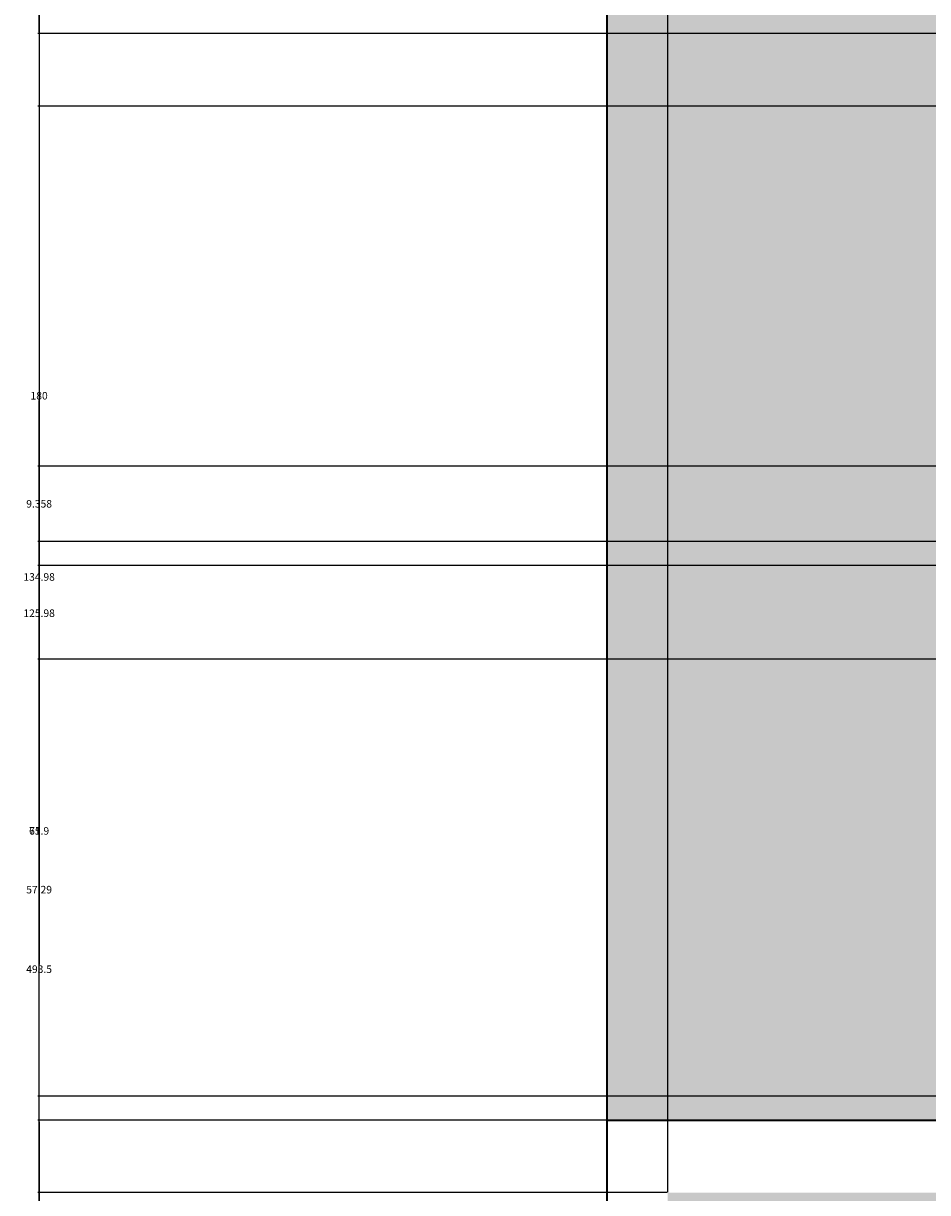
# Model space of a CAD drawing. Units: inches. Extents: x -5 to 714, y 84 to 644.
# Tile 7 of 20: x -5 to 108, y 336 to 481. Entities that reach past the tile are written whole.
import ezdxf

# ---------------------------------------------------------------- set-up
doc = ezdxf.new("R2010")
doc.units = ezdxf.units.IN
doc.header["$MEASUREMENT"] = 0
for name, color, linetype, lineweight in [('A-ANNO-DIMS', 2, 'Continuous', 18), ('A-ELEV', 7, 'Continuous', 35), ('A-ELEV-PATT', 8, 'Continuous', 13)]:
    doc.layers.add(name, color=color, linetype=linetype, lineweight=lineweight)
doc.styles.get("Standard").update_dxf_attribs({"font": 'arial.ttf'})
doc.dimstyles.get("Standard").update_dxf_attribs({"dimtxt": 0.9375, "dimasz": 0.18, "dimexe": 0.18, "dimexo": 0.0625, "dimgap": 0.09, "dimtad": 0, "dimtih": 1, "dimtoh": 1, "dimdec": 4, "dimzin": 0, "dimdsep": 46, "dimlunit": 4, "dimtxsty": 'Standard', "dimcen": 0.09, "dimadec": 0, "dimazin": 0, "dimtfac": 1, "dimtdec": 4, "dimtofl": 0, "dimtmove": 0, "dimatfit": 3, "dimfxl": 1, "dimtolj": 1, "dimtzin": 0, "dimarcsym": 0})

# ---------------------------------------------------------------- blocks, each defined once
blk = doc.blocks.new('*D2')
at = {"layer": 'A-ANNO-DIMS', "color": 0, "lineweight": -2, "transparency": 16777216}
for p, q in [((67.93, 610.73), (-2.74, 610.73)), ((-2.56, 610.55), (-2.56, 364.53)), ((-2.56, 117.37), (-2.56, 363.39)), ((30.08, 117.19), (-2.74, 117.19))]:
    blk.add_line(p, q, dxfattribs=at)
at = {"layer": 'A-ANNO-DIMS', "color": 0, "transparency": 16777216}
for points in [[(-2.59, 610.55), (-2.53, 610.55), (-2.56, 610.73)], [(-2.59, 117.37), (-2.53, 117.37), (-2.56, 117.19)]]:
    blk.add_solid(points, dxfattribs=at)
at = {"layer": 'Defpoints', "color": 0, "transparency": 16777216}
for p in [(-2.56, 610.73), (67.99, 610.73), (30.14, 117.19)]:
    blk.add_point(p, dxfattribs=at)
at = {"layer": 'A-ANNO-DIMS', "color": 0, "transparency": 16777216, "insert": (-2.56, 363.96), "char_height": 0.938, "attachment_point": 5}
blk.add_mtext('\\A1;493.5', dxfattribs=at)
blk = doc.blocks.new('*D5')
at = {"layer": 'A-ANNO-DIMS', "color": 0, "lineweight": -2, "transparency": 16777216}
for p, q in [((67.93, 345.19), (-2.74, 345.19)), ((-2.56, 345.01), (-2.56, 273.75)), ((-2.56, 201.37), (-2.56, 272.63)), ((67.93, 201.19), (-2.74, 201.19))]:
    blk.add_line(p, q, dxfattribs=at)
at = {"layer": 'A-ANNO-DIMS', "color": 0, "transparency": 16777216}
for points in [[(-2.59, 345.01), (-2.53, 345.01), (-2.56, 345.19)], [(-2.59, 201.37), (-2.53, 201.37), (-2.56, 201.19)]]:
    blk.add_solid(points, dxfattribs=at)
at = {"layer": 'Defpoints', "color": 0, "transparency": 16777216}
for p in [(-2.56, 345.19), (67.99, 345.19), (67.99, 201.19)]:
    blk.add_point(p, dxfattribs=at)
at = {"layer": 'A-ANNO-DIMS', "color": 0, "transparency": 16777216, "insert": (-2.56, 273.19), "char_height": 0.938, "attachment_point": 5}
blk.add_mtext('\\A1;144', dxfattribs=at)
blk = doc.blocks.new('*D6')
at = {"layer": 'A-ANNO-DIMS', "color": 0, "lineweight": -2, "transparency": 16777216}
for p, q in [((67.93, 525.19), (-2.74, 525.19)), ((-2.56, 525.01), (-2.56, 435.76)), ((-2.56, 345.37), (-2.56, 434.62)), ((67.93, 345.19), (-2.74, 345.19))]:
    blk.add_line(p, q, dxfattribs=at)
at = {"layer": 'A-ANNO-DIMS', "color": 0, "transparency": 16777216}
for points in [[(-2.59, 525.01), (-2.53, 525.01), (-2.56, 525.19)], [(-2.59, 345.37), (-2.53, 345.37), (-2.56, 345.19)]]:
    blk.add_solid(points, dxfattribs=at)
at = {"layer": 'Defpoints', "color": 0, "transparency": 16777216}
for p in [(-2.56, 525.19), (67.99, 525.19), (67.99, 345.19)]:
    blk.add_point(p, dxfattribs=at)
at = {"layer": 'A-ANNO-DIMS', "color": 0, "transparency": 16777216, "insert": (-2.56, 435.19), "char_height": 0.938, "attachment_point": 5}
blk.add_mtext('\\A1;180', dxfattribs=at)
blk = doc.blocks.new('*D16')
at = {"layer": 'A-ANNO-DIMS', "color": 0, "lineweight": -2, "transparency": 16777216}
for p, q in [((364.22, 540.29), (-2.74, 540.29)), ((-2.56, 540.11), (-2.56, 510.8)), ((-2.56, 480.35), (-2.56, 509.66)), ((364.22, 480.17), (-2.74, 480.17))]:
    blk.add_line(p, q, dxfattribs=at)
at = {"layer": 'A-ANNO-DIMS', "color": 0, "transparency": 16777216}
for points in [[(-2.59, 540.11), (-2.53, 540.11), (-2.56, 540.29)], [(-2.59, 480.35), (-2.53, 480.35), (-2.56, 480.17)]]:
    blk.add_solid(points, dxfattribs=at)
at = {"layer": 'Defpoints', "color": 0, "transparency": 16777216}
for p in [(-2.56, 540.29), (364.28, 540.29), (364.28, 480.17)]:
    blk.add_point(p, dxfattribs=at)
at = {"layer": 'A-ANNO-DIMS', "color": 0, "transparency": 16777216, "insert": (-2.56, 510.23), "char_height": 0.938, "attachment_point": 5}
blk.add_mtext('\\A1;60.11', dxfattribs=at)
blk = doc.blocks.new('*D23')
at = {"layer": 'A-ANNO-DIMS', "color": 0, "lineweight": -2, "transparency": 16777216}
for p, q in [((229.3, 525.19), (-2.74, 525.19)), ((-2.56, 525.01), (-2.56, 503.25)), ((-2.56, 480.35), (-2.56, 502.11)), ((229.3, 480.17), (-2.74, 480.17))]:
    blk.add_line(p, q, dxfattribs=at)
at = {"layer": 'A-ANNO-DIMS', "color": 0, "transparency": 16777216}
for points in [[(-2.59, 525.01), (-2.53, 525.01), (-2.56, 525.19)], [(-2.59, 480.35), (-2.53, 480.35), (-2.56, 480.17)]]:
    blk.add_solid(points, dxfattribs=at)
at = {"layer": 'Defpoints', "color": 0, "transparency": 16777216}
for p in [(-2.56, 525.19), (229.36, 525.19), (229.36, 480.17)]:
    blk.add_point(p, dxfattribs=at)
at = {"layer": 'A-ANNO-DIMS', "color": 0, "transparency": 16777216, "insert": (-2.56, 502.68), "char_height": 0.938, "attachment_point": 5}
blk.add_mtext('\\A1;45.02', dxfattribs=at)
blk = doc.blocks.new('*D25')
at = {"layer": 'A-ANNO-DIMS', "color": 0, "lineweight": -2, "transparency": 16777216}
for p, q in [((126.67, 480.17), (-2.74, 480.17)), ((-2.56, 479.99), (-2.56, 413.25)), ((-2.56, 345.37), (-2.56, 412.11)), ((126.67, 345.19), (-2.74, 345.19))]:
    blk.add_line(p, q, dxfattribs=at)
at = {"layer": 'A-ANNO-DIMS', "color": 0, "transparency": 16777216}
for points in [[(-2.59, 479.99), (-2.53, 479.99), (-2.56, 480.17)], [(-2.59, 345.37), (-2.53, 345.37), (-2.56, 345.19)]]:
    blk.add_solid(points, dxfattribs=at)
at = {"layer": 'Defpoints', "color": 0, "transparency": 16777216}
for p in [(-2.56, 480.17), (126.73, 480.17), (126.73, 345.19)]:
    blk.add_point(p, dxfattribs=at)
at = {"layer": 'A-ANNO-DIMS', "color": 0, "transparency": 16777216, "insert": (-2.56, 412.68), "char_height": 0.938, "attachment_point": 5}
blk.add_mtext('\\A1;134.98', dxfattribs=at)
blk = doc.blocks.new('*D26')
at = {"layer": 'A-ANNO-DIMS', "color": 0, "lineweight": -2, "transparency": 16777216}
for p, q in [((135.67, 471.17), (-2.74, 471.17)), ((-2.56, 470.99), (-2.56, 408.75)), ((-2.56, 345.37), (-2.56, 407.61)), ((135.67, 345.19), (-2.74, 345.19))]:
    blk.add_line(p, q, dxfattribs=at)
at = {"layer": 'A-ANNO-DIMS', "color": 0, "transparency": 16777216}
for points in [[(-2.59, 470.99), (-2.53, 470.99), (-2.56, 471.17)], [(-2.59, 345.37), (-2.53, 345.37), (-2.56, 345.19)]]:
    blk.add_solid(points, dxfattribs=at)
at = {"layer": 'Defpoints', "color": 0, "transparency": 16777216}
for p in [(-2.56, 471.17), (135.73, 471.17), (135.73, 345.19)]:
    blk.add_point(p, dxfattribs=at)
at = {"layer": 'A-ANNO-DIMS', "color": 0, "transparency": 16777216, "insert": (-2.56, 408.18), "char_height": 0.938, "attachment_point": 5}
blk.add_mtext('\\A1;125.98', dxfattribs=at)
blk = doc.blocks.new('*D27')
at = {"layer": 'A-ANNO-DIMS', "color": 0, "lineweight": -2, "transparency": 16777216}
for p, q in [((429.45, 402.48), (-2.74, 402.48)), ((-2.56, 402.3), (-2.56, 374.41)), ((-2.56, 345.37), (-2.56, 373.27)), ((429.45, 345.19), (-2.74, 345.19))]:
    blk.add_line(p, q, dxfattribs=at)
at = {"layer": 'A-ANNO-DIMS', "color": 0, "transparency": 16777216}
for points in [[(-2.59, 402.3), (-2.53, 402.3), (-2.56, 402.48)], [(-2.59, 345.37), (-2.53, 345.37), (-2.56, 345.19)]]:
    blk.add_solid(points, dxfattribs=at)
at = {"layer": 'Defpoints', "color": 0, "transparency": 16777216}
for p in [(-2.56, 402.48), (429.51, 402.48), (429.51, 345.19)]:
    blk.add_point(p, dxfattribs=at)
at = {"layer": 'A-ANNO-DIMS', "color": 0, "transparency": 16777216, "insert": (-2.56, 373.84), "char_height": 0.938, "attachment_point": 5}
blk.add_mtext('\\A1;57.29', dxfattribs=at)
blk = doc.blocks.new('*D34')
at = {"layer": 'A-ANNO-DIMS', "color": 0, "lineweight": -2, "transparency": 16777216}
for p, q in [((286.82, 414.09), (-2.74, 414.09)), ((-2.56, 413.91), (-2.56, 381.71)), ((-2.56, 348.37), (-2.56, 380.57)), ((286.82, 348.19), (-2.74, 348.19))]:
    blk.add_line(p, q, dxfattribs=at)
at = {"layer": 'A-ANNO-DIMS', "color": 0, "transparency": 16777216}
for points in [[(-2.59, 413.91), (-2.53, 413.91), (-2.56, 414.09)], [(-2.59, 348.37), (-2.53, 348.37), (-2.56, 348.19)]]:
    blk.add_solid(points, dxfattribs=at)
at = {"layer": 'Defpoints', "color": 0, "transparency": 16777216}
for p in [(-2.56, 414.09), (286.88, 414.09), (286.88, 348.19)]:
    blk.add_point(p, dxfattribs=at)
at = {"layer": 'A-ANNO-DIMS', "color": 0, "transparency": 16777216, "insert": (-2.56, 381.14), "char_height": 0.938, "attachment_point": 5}
blk.add_mtext('\\A1;65.9', dxfattribs=at)
blk = doc.blocks.new('*D35')
at = {"layer": 'A-ANNO-DIMS', "color": 0, "lineweight": -2, "transparency": 16777216}
for p, q in [((289.82, 417.09), (-2.74, 417.09)), ((-2.56, 416.91), (-2.56, 381.71)), ((-2.56, 345.37), (-2.56, 380.57)), ((289.82, 345.19), (-2.74, 345.19))]:
    blk.add_line(p, q, dxfattribs=at)
at = {"layer": 'A-ANNO-DIMS', "color": 0, "transparency": 16777216}
for points in [[(-2.59, 416.91), (-2.53, 416.91), (-2.56, 417.09)], [(-2.59, 345.37), (-2.53, 345.37), (-2.56, 345.19)]]:
    blk.add_solid(points, dxfattribs=at)
at = {"layer": 'Defpoints', "color": 0, "transparency": 16777216}
for p in [(-2.56, 417.09), (289.88, 417.09), (289.88, 345.19)]:
    blk.add_point(p, dxfattribs=at)
at = {"layer": 'A-ANNO-DIMS', "color": 0, "transparency": 16777216, "insert": (-2.56, 381.14), "char_height": 0.938, "attachment_point": 5}
blk.add_mtext('\\A1;71.9', dxfattribs=at)
blk = doc.blocks.new('*D37')
at = {"layer": 'A-ANNO-DIMS', "color": 0, "lineweight": -2, "transparency": 16777216}
for p, q in [((302.44, 426.45), (-2.74, 426.45)), ((-2.56, 426.27), (-2.56, 422.34)), ((-2.56, 417.27), (-2.56, 421.2)), ((302.44, 417.09), (-2.74, 417.09))]:
    blk.add_line(p, q, dxfattribs=at)
at = {"layer": 'A-ANNO-DIMS', "color": 0, "transparency": 16777216}
for points in [[(-2.59, 426.27), (-2.53, 426.27), (-2.56, 426.45)], [(-2.59, 417.27), (-2.53, 417.27), (-2.56, 417.09)]]:
    blk.add_solid(points, dxfattribs=at)
at = {"layer": 'Defpoints', "color": 0, "transparency": 16777216}
for p in [(-2.56, 426.45), (302.5, 426.45), (302.5, 417.09)]:
    blk.add_point(p, dxfattribs=at)
at = {"layer": 'A-ANNO-DIMS', "color": 0, "transparency": 16777216, "insert": (-2.56, 421.77), "char_height": 0.938, "attachment_point": 5}
blk.add_mtext('\\A1;9.358', dxfattribs=at)
blk = doc.blocks.new('*D45')
at = {"layer": 'A-ANNO-DIMS', "color": 0, "lineweight": -2, "transparency": 16777216}
for p, q in [((75.44, 336.21), (-2.74, 336.21)), ((-2.56, 336.03), (-2.56, 328.34)), ((-2.56, 319.52), (-2.56, 327.21)), ((75.44, 319.34), (-2.74, 319.34))]:
    blk.add_line(p, q, dxfattribs=at)
at = {"layer": 'A-ANNO-DIMS', "color": 0, "transparency": 16777216}
for points in [[(-2.59, 336.03), (-2.53, 336.03), (-2.56, 336.21)], [(-2.59, 319.52), (-2.53, 319.52), (-2.56, 319.34)]]:
    blk.add_solid(points, dxfattribs=at)
at = {"layer": 'Defpoints', "color": 0, "transparency": 16777216}
for p in [(-2.56, 336.21), (75.5, 336.21), (75.5, 319.34)]:
    blk.add_point(p, dxfattribs=at)
at = {"layer": 'A-ANNO-DIMS', "color": 0, "transparency": 16777216, "insert": (-2.56, 327.78), "char_height": 0.938, "attachment_point": 5}
blk.add_mtext('\\A1;16.86', dxfattribs=at)
blk = doc.blocks.new('*D46')
at = {"layer": 'A-ANNO-DIMS', "color": 0, "lineweight": -2, "transparency": 16777216}
for p, q in [((67.99, 345.26), (67.99, 643.61)), ((68.17, 643.43), (70.08, 643.43)), ((75.32, 643.43), (73.41, 643.43)), ((75.5, 336.27), (75.5, 643.61))]:
    blk.add_line(p, q, dxfattribs=at)
at = {"layer": 'A-ANNO-DIMS', "color": 0, "transparency": 16777216}
for points in [[(68.17, 643.46), (68.17, 643.4), (67.99, 643.43)], [(75.32, 643.46), (75.32, 643.4), (75.5, 643.43)]]:
    blk.add_solid(points, dxfattribs=at)
at = {"layer": 'Defpoints', "color": 0, "transparency": 16777216}
for p in [(75.5, 643.43), (67.99, 345.19), (75.5, 336.21)]:
    blk.add_point(p, dxfattribs=at)
at = {"layer": 'A-ANNO-DIMS', "color": 0, "transparency": 16777216, "insert": (71.75, 643.43), "char_height": 0.938, "attachment_point": 5}
blk.add_mtext('\\A1;7.516', dxfattribs=at)
blk = doc.blocks.new('*D47')
at = {"layer": 'A-ANNO-DIMS', "color": 0, "lineweight": -2, "transparency": 16777216}
for p, q in [((75.5, 336.27), (75.5, 643.61)), ((75.68, 643.43), (96.74, 643.43)), ((121.18, 643.43), (100.13, 643.43)), ((121.36, 336.27), (121.36, 643.61))]:
    blk.add_line(p, q, dxfattribs=at)
at = {"layer": 'A-ANNO-DIMS', "color": 0, "transparency": 16777216}
for points in [[(75.68, 643.46), (75.68, 643.4), (75.5, 643.43)], [(121.18, 643.46), (121.18, 643.4), (121.36, 643.43)]]:
    blk.add_solid(points, dxfattribs=at)
at = {"layer": 'Defpoints', "color": 0, "transparency": 16777216}
for p in [(121.36, 643.43), (75.5, 336.21), (121.36, 336.21)]:
    blk.add_point(p, dxfattribs=at)
at = {"layer": 'A-ANNO-DIMS', "color": 0, "transparency": 16777216, "insert": (98.43, 643.43), "char_height": 0.938, "attachment_point": 5}
blk.add_mtext('\\A1;45.85', dxfattribs=at)
blk = doc.blocks.new('*D50')
at = {"layer": 'A-ANNO-DIMS', "color": 0, "lineweight": -2, "transparency": 16777216}
for p, q in [((200.67, 345.19), (-2.74, 345.19)), ((-2.56, 345.01), (-2.56, 324.13)), ((-2.56, 302.12), (-2.56, 323)), ((200.67, 301.94), (-2.74, 301.94))]:
    blk.add_line(p, q, dxfattribs=at)
at = {"layer": 'A-ANNO-DIMS', "color": 0, "transparency": 16777216}
for points in [[(-2.59, 345.01), (-2.53, 345.01), (-2.56, 345.19)], [(-2.59, 302.12), (-2.53, 302.12), (-2.56, 301.94)]]:
    blk.add_solid(points, dxfattribs=at)
at = {"layer": 'Defpoints', "color": 0, "transparency": 16777216}
for p in [(-2.56, 345.19), (200.74, 345.19), (200.74, 301.94)]:
    blk.add_point(p, dxfattribs=at)
at = {"layer": 'A-ANNO-DIMS', "color": 0, "transparency": 16777216, "insert": (-2.56, 323.57), "char_height": 0.938, "attachment_point": 5}
blk.add_mtext('\\A1;43.255', dxfattribs=at)

msp = doc.modelspace()

# ---------------------------------------------------------------- hatches: boundary and pattern name
at = {"layer": 'A-ELEV-PATT', "transparency": 33554687}
h = msp.add_hatch(color=256, dxfattribs=at)
h.dxf.hatch_style = 1
h.paths.add_polyline_path([(188.3677, 525.1928), (67.9893, 525.1928), (67.9893, 489.1928), (67.9893, 345.1928), (126.7303, 345.1928), (126.7303, 480.1709), (229.3575, 480.1709), (229.3575, 525.1928), (212.6043, 525.1928), (212.6043, 482.7164), (211.0019, 482.7164), (211.0019, 525.1928), (207.6919, 525.1928), (199.9852, 525.1928), (199.9852, 482.7164), (198.3828, 482.7164), (198.3828, 525.1928), (189.9701, 525.1928), (189.9701, 482.7164), (188.3677, 482.7164)])
h.paths.add_polyline_path([(121.3589, 336.2066), (75.5048, 336.2066), (75.5048, 319.345), (121.3589, 319.345)])
h.paths.add_polyline_path([(121.3589, 319.345), (75.5048, 319.345), (75.5048, 302.3045), (121.3589, 302.3045)])
h.paths.add_polyline_path([(121.3589, 302.3045), (75.5048, 302.3045), (75.5048, 282.8561), (121.3589, 282.8561)])
h.paths.add_polyline_path([(121.3589, 282.8561), (75.5048, 282.8561), (75.5048, 261.5556), (121.3589, 261.5556)])
h.paths.add_polyline_path([(121.3589, 261.5556), (75.5048, 261.5556), (75.5048, 243.7009), (121.3589, 243.7009)])
h.paths.add_polyline_path([(121.3589, 243.7009), (75.5048, 243.7009), (75.5048, 223.5117), (121.3589, 223.5117)])
h.paths.add_polyline_path([(121.3589, 223.5117), (75.5048, 223.5117), (75.5048, 212.5836), (121.3589, 212.5836)])
h.paths.add_polyline_path([(121.3589, 212.5836), (75.5048, 212.5836), (75.5048, 201.1928), (121.3589, 201.1928)])
h.paths.add_polyline_path([(179.9335, 201.1928), (30.1395, 201.1928), (30.1395, 198.7054), (179.9335, 198.7054)])
h.paths.add_polyline_path([(187.6349, 201.1928), (179.9335, 201.1928), (179.9335, 198.7054), (179.9335, 141.1928), (269.2446, 141.1928), (269.2446, 201.1928), (263.4349, 201.1928), (263.4349, 152.1176), (187.6349, 152.1176)])
h.paths.add_polyline_path([(269.2446, 277.0513), (269.2446, 287.501), (269.2446, 306.6286), (578.0915, 306.6286), (578.0915, 201.1928), (593.428, 201.1928), (593.428, 315.0968), (584.4202, 315.0968), (259.0665, 315.0968), (259.0665, 201.1928), (263.4349, 201.1928), (269.2446, 201.1928)])

# ---------------------------------------------------------------- linework, layer by layer
at = {"layer": 'A-ELEV'}
for p, q in [((67.9893, 345.1928), (67.9893, 489.1928)), ((67.9893, 201.1928), (67.9893, 345.1928)), ((67.9893, 345.1928), (587.5794, 345.1928))]:
    msp.add_line(p, q, dxfattribs=at)

# ---------------------------------------------------------------- dimensions: what is measured, and where the dimension line sits
at = {"layer": 'A-ANNO-DIMS'}
for base, p1, p2, override, picture, middle in [((75.50483, 643.42757), (67.9893, 345.19283), (75.50483, 336.20661), {"dimdec": 3, "dimlfac": 1, "dimrnd": 0, "dimzin": 0, "dimdsep": 46, "dimlunit": 2}, '*D46', (71.74706, 643.42757)), ((121.3589, 643.4276), (75.5048, 336.2066), (121.3589, 336.2066), {"dimdec": 2, "dimlfac": 1, "dimrnd": 0, "dimzin": 0, "dimdsep": 46, "dimlunit": 2}, '*D47', (98.4319, 643.4276))]:
    dim = msp.add_linear_dim(base=base, p1=p1, p2=p2, dimstyle='Standard', override=override, dxfattribs=at)
    dim.commit()
    dim.dimension.update_dxf_attribs({"geometry": picture, "text_midpoint": middle})
for base, p1, p2, override, picture, middle in [((-2.5605, 610.7276), (30.1395, 117.1928), (67.9893, 610.7276), {"dimdec": 1, "dimlfac": 1, "dimrnd": 0, "dimzin": 0, "dimdsep": 46, "dimlunit": 2}, '*D2', (-2.5605, 363.9602)), ((-2.5605, 540.2857), (364.2809, 480.1709), (364.2809, 540.2857), {"dimdec": 2, "dimlfac": 1, "dimrnd": 0, "dimzin": 0, "dimdsep": 46, "dimlunit": 2}, '*D16', (-2.5605, 510.2283)), ((-2.5605, 525.1928), (229.3575, 480.1709), (229.3575, 525.1928), {"dimdec": 2, "dimlfac": 1, "dimrnd": 0, "dimzin": 0, "dimdsep": 46, "dimlunit": 2}, '*D23', (-2.5605, 502.6819)), ((-2.5605, 525.1928), (67.9893, 345.1928), (67.9893, 525.1928), {"dimdec": 0, "dimlfac": 1, "dimrnd": 0, "dimzin": 0, "dimdsep": 46, "dimlunit": 2}, '*D6', (-2.5605, 435.1928)), ((-2.5605, 480.1709), (126.7303, 345.1928), (126.7303, 480.1709), {"dimdec": 2, "dimlfac": 1, "dimrnd": 0, "dimzin": 0, "dimdsep": 46, "dimlunit": 2}, '*D25', (-2.5605, 412.6819)), ((-2.5605, 471.1709), (135.7303, 345.1928), (135.7303, 471.1709), {"dimdec": 2, "dimlfac": 1, "dimrnd": 0, "dimzin": 0, "dimdsep": 46, "dimlunit": 2}, '*D26', (-2.5605, 408.1819)), ((-2.5605, 426.4485), (302.5023, 417.0908), (302.5023, 426.4485), {"dimdec": 3, "dimlfac": 1, "dimrnd": 0, "dimzin": 0, "dimdsep": 46, "dimlunit": 2}, '*D37', (-2.5605, 421.7696)), ((-2.5605, 417.0908), (289.8815, 345.1928), (289.8815, 417.0908), {"dimdec": 1, "dimlfac": 1, "dimrnd": 0, "dimzin": 0, "dimdsep": 46, "dimlunit": 2}, '*D35', (-2.5605, 381.1418)), ((-2.5605, 414.0908), (286.8815, 348.1928), (286.8815, 414.0908), {"dimdec": 1, "dimlfac": 1, "dimrnd": 0, "dimzin": 0, "dimdsep": 46, "dimlunit": 2}, '*D34', (-2.5605, 381.1418)), ((-2.5605, 402.4806), (429.5094, 345.1928), (429.5094, 402.4806), {"dimdec": 2, "dimlfac": 1, "dimrnd": 0, "dimzin": 0, "dimdsep": 46, "dimlunit": 2}, '*D27', (-2.5605, 373.8367)), ((-2.5605, 345.1928), (200.7361, 301.9374), (200.7361, 345.1928), {"dimdec": 3, "dimlfac": 1, "dimrnd": 0, "dimzin": 0, "dimdsep": 46, "dimlunit": 2}, '*D50', (-2.5605, 323.5651)), ((-2.5605, 345.1928), (67.9893, 201.1928), (67.9893, 345.1928), {"dimdec": 0, "dimlfac": 1, "dimrnd": 0, "dimzin": 0, "dimdsep": 46, "dimlunit": 2}, '*D5', (-2.5605, 273.1928)), ((-2.5605, 336.2066), (75.5048, 319.345), (75.5048, 336.2066), {"dimdec": 2, "dimlfac": 1, "dimrnd": 0, "dimzin": 0, "dimdsep": 46, "dimlunit": 2}, '*D45', (-2.5605, 327.7758))]:
    dim = msp.add_linear_dim(base=base, p1=p1, p2=p2, angle=90, dimstyle='Standard', override=override, dxfattribs=at)
    dim.commit()
    dim.dimension.update_dxf_attribs({"geometry": picture, "text_midpoint": middle})

doc.saveas('drawing.dxf')
